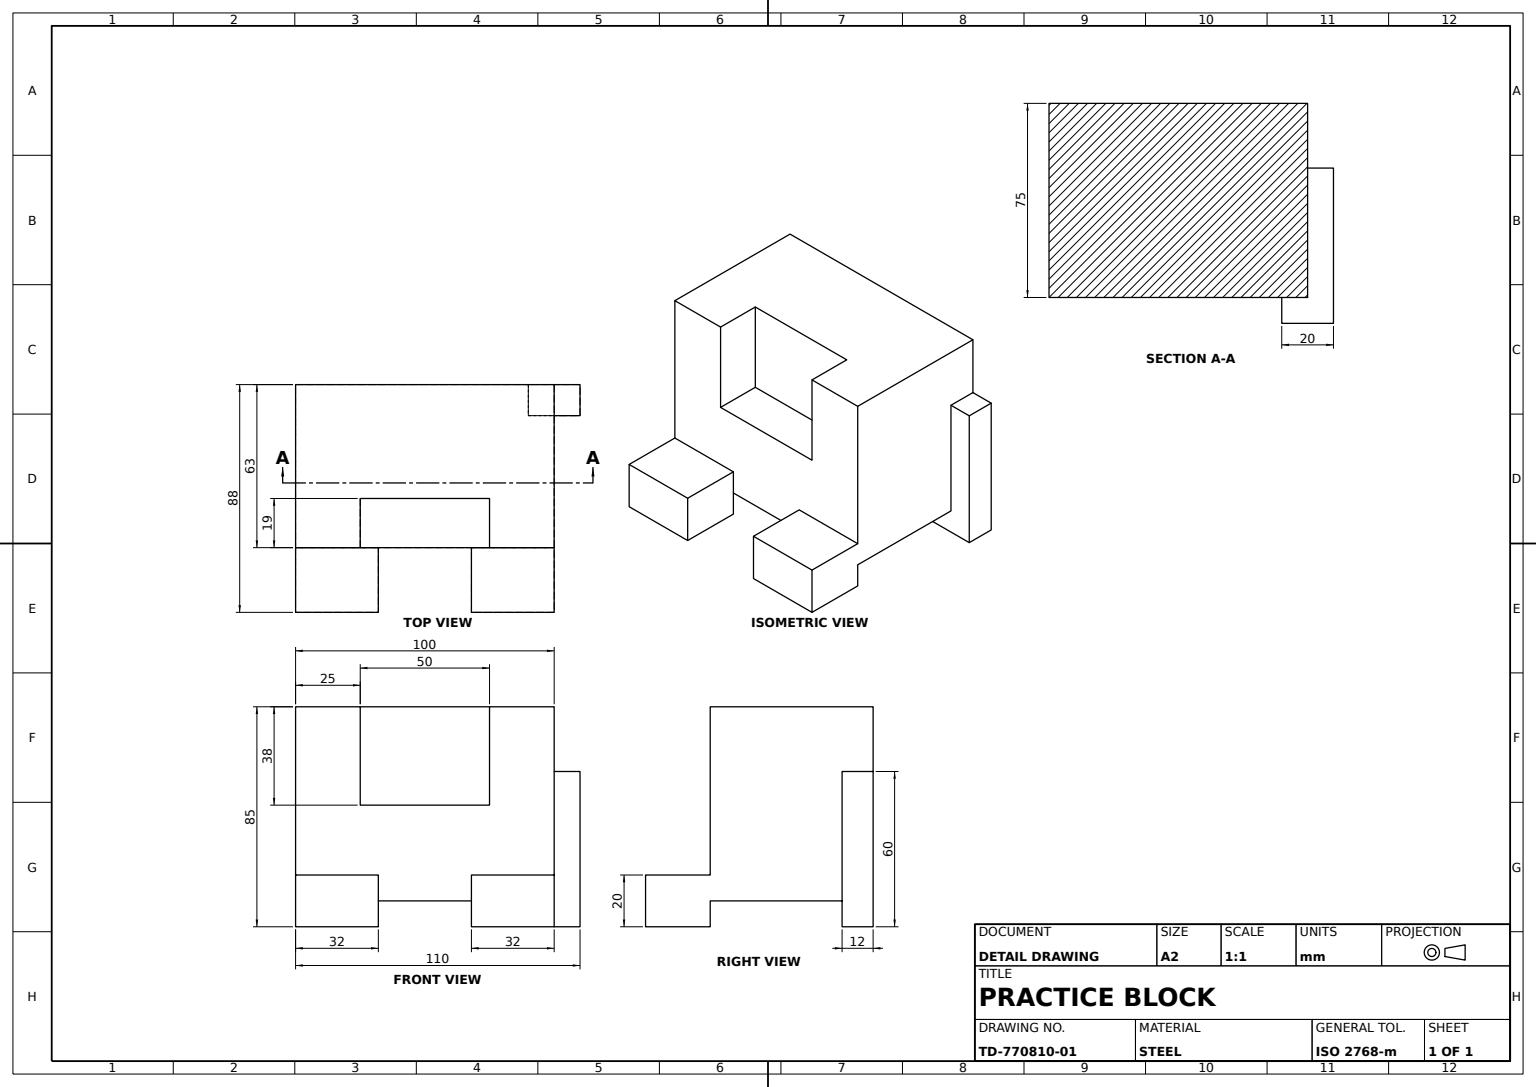
from build123d import *

# Parameters (mm, degrees)
BASE_BLOCK_SKETCH_W        = 100
BASE_BLOCK_SKETCH_H        = 63
BASE_BLOCK_100X63X75_DEPTH = 75
TOP_POCKET_SKETCH_W        = 50
TOP_POCKET_SKETCH_H        = 38
TOP_POCKET_38X25X19_DEPTH  = 19
FEET_SKETCH_W              = 32
FEET_SKETCH_H              = 25
FEET_2X_32X25_DEPTH        = 10
SIDE_RIB_DEPTH             = 10


with BuildPart() as part:
    # Base Block Sketch → Base Block 100x63x75 (new body)
    with BuildSketch(Plane(origin=(0, 0, 0), x_dir=(1, 0, 0), z_dir=(0, 1, 0))):
        with Locations((50, 31.5)):
            Rectangle(BASE_BLOCK_SKETCH_W, BASE_BLOCK_SKETCH_H)
    extrude(amount=BASE_BLOCK_100X63X75_DEPTH)

    # Top Pocket Sketch → Top Pocket 38x25x19 (cut)
    with BuildSketch(Plane.XY):
        with Locations((50, 56)):
            Rectangle(TOP_POCKET_SKETCH_W, TOP_POCKET_SKETCH_H)
    extrude(amount=-TOP_POCKET_38X25X19_DEPTH, mode=Mode.SUBTRACT)

    # Feet Sketch → Feet 2x 32x25 (add, symmetric)
    with BuildSketch(Plane.XZ):
        with Locations((16, 12.5)):
            Rectangle(FEET_SKETCH_W, FEET_SKETCH_H)
        with Locations((84, 12.5)):
            Rectangle(FEET_SKETCH_W, FEET_SKETCH_H)
    extrude(amount=FEET_2X_32X25_DEPTH, both=True)

    # Side Rib Sketch → Side Rib (add, symmetric)
    with BuildSketch(Plane(origin=(100, 0, 0), x_dir=(0, 0, -1), z_dir=(1, 0, 0))):
        Polygon((63, 0), (63, 50), (51, 50), (51, -10), (63, -10), align=None)
    extrude(amount=SIDE_RIB_DEPTH, both=True)


solid = part.part
